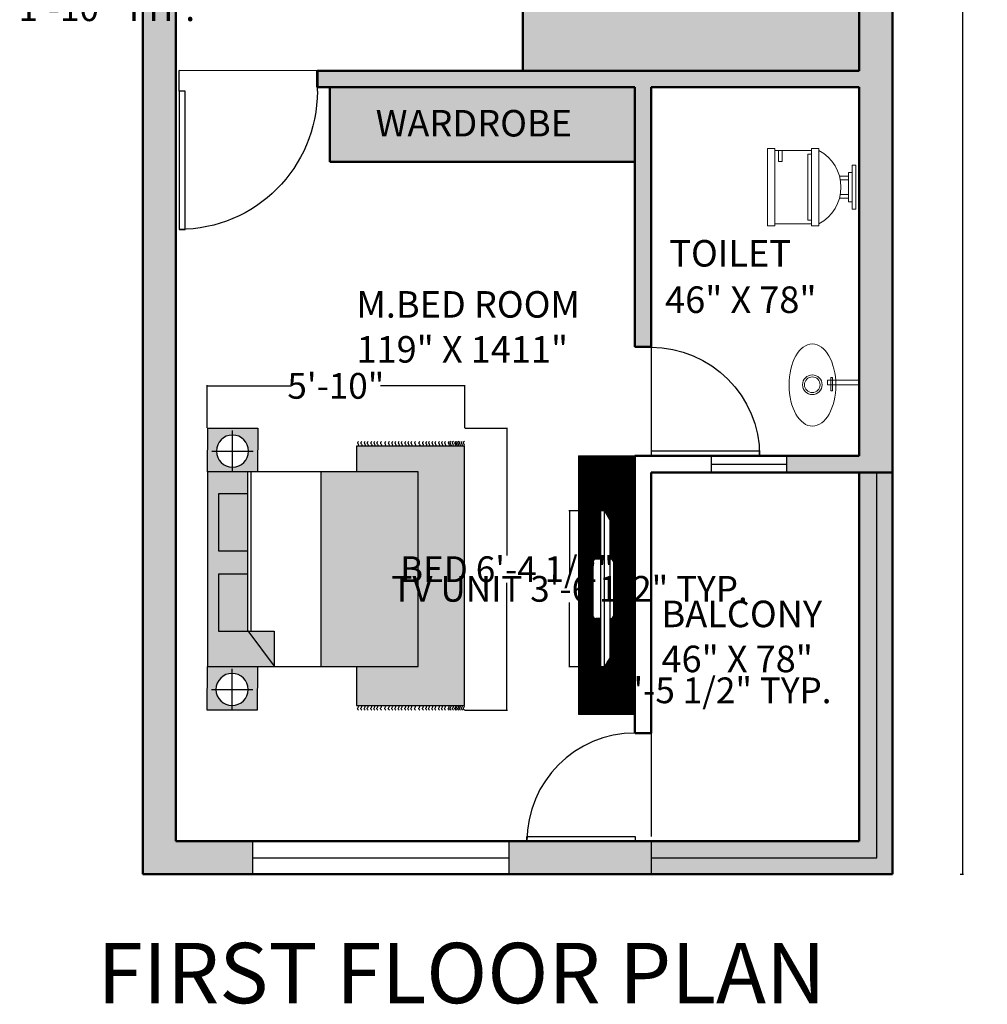
# Model space of a CAD drawing. Units: inches. Extents: x 679 to 1269, y 101 to 755.
# Tile 2 of 6: x 952 to 1216, y 102 to 370. Entities that reach past the tile are written whole.
import ezdxf

# ---------------------------------------------------------------- set-up
doc = ezdxf.new("R2010")
doc.units = ezdxf.units.IN
doc.header["$MEASUREMENT"] = 0
for name, color, linetype, lineweight in [('A-ANNO-DIMS', 2, 'Continuous', 18), ('A-ANNO-TEXT', 7, 'Continuous', 25), ('A-AREA-IDEN', 7, 'Continuous', 25), ('A-DOOR', 4, 'Continuous', 25), ('A-FLOR-FIXT', 8, 'Continuous', 18), ('A-FLOR-PATT', 8, 'Continuous', 13), ('A-FURN', 32, 'Continuous', 18), ('A-FURN-PATT', 252, 'Continuous', 13), ('A-GLAZ', 4, 'Continuous', 25), ('A-WALL', 7, 'Continuous', 50), ('A-WALL-PATT', 8, 'Continuous', 13)]:
    doc.layers.add(name, color=color, linetype=linetype, lineweight=lineweight)
doc.layers.add('furniture', color=32, linetype='Continuous')
doc.styles.get("Standard").update_dxf_attribs({"font": 'arial.ttf'})
doc.dimstyles.get("Standard").update_dxf_attribs({"dimtxt": 7, "dimasz": 0.18, "dimexe": 0.18, "dimexo": 0.0625, "dimgap": 0.09, "dimtad": 0, "dimtih": 1, "dimtoh": 1, "dimzin": 0, "dimdsep": 46, "dimlunit": 3, "dimtxsty": 'Standard', "dimcen": 0.09, "dimadec": 0, "dimazin": 0, "dimtfac": 1, "dimtofl": 0, "dimtmove": 0, "dimatfit": 3, "dimfxl": 1, "dimtolj": 1, "dimtzin": 0, "dimarcsym": 0})

# ---------------------------------------------------------------- blocks, each defined once
blk = doc.blocks.new('*U12')
for p, q in [((-10, 22), (-10, 12)), ((10, 12), (10, 22)), ((-10, 21), (-7, 21)), ((-7, 20), (-10, 20)), ((-7, 21), (-7, 20)), ((10.5, 12), (-10.5, 12)), ((-10.5, 10), (-10.5, 12)), ((9, 13), (-9, 13)), ((-9, 13), (-9, 12)), ((9, 12), (9, 13)), ((10.5, 12), (10.5, 10)), ((10.5, 10), (-10.5, 10)), ((-3, 4.4065), (-3, 2)), ((-2, 2), (-2, 4.1658)), ((2, 4.1658), (2, 2)), ((3, 2), (3, 4.4065)), ((4, 2), (-4, 2)), ((-4, 2), (-4, 1)), ((4, 1), (4, 2))]:
    blk.add_line(p, q)
for points in [[(10.5, 22), (10.5, 24), (-10.5, 24), (-10.5, 22)], [(6, 0), (6, 1), (-6, 1), (-6, 0)]]:
    blk.add_lwpolyline(points, close=True)
blk.add_arc((0, 15.3333), 11.3333, 208.0725, 331.9275)
blk = doc.blocks.new('PLASMA-LARGE')
at = {"layer": 'furniture'}
for p, q in [((-7.26, 0), (7.26, 0)), ((-21, -2.5), (21, -2.5)), ((-21, -2.5), (-21, -3.5)), ((-18.61, -1), (18.61, -1)), ((-8, -1), (-8, -0.74)), ((8, -1), (8, -0.74)), ((21, -2.5), (21, -3.5)), ((-21, -3.5), (21, -3.5)), ((-8, -3.5), (-8, -4.76)), ((8, -3.5), (8, -4.76)), ((-7.26, -5.5), (7.26, -5.5))]:
    blk.add_line(p, q, dxfattribs=at)
for centre, radius, start, end in [((-7.26, -0.74), 0.744, 90, 180), ((7.26, -0.74), 0.744, 0, 90), ((-13.97, -11.05), 11.07, 114.7602, 129.4175), ((13.97, -11.05), 11.07, 50.5825, 65.2398), ((-7.26, -4.76), 0.744, 180, 270), ((7.26, -4.76), 0.744, 270, 0)]:
    blk.add_arc(centre, radius, start, end, dxfattribs=at)
blk = doc.blocks.new('CARPET')
at = {"layer": 'furniture'}
for p, q in [((-51.53, -98.11), (-51.53, -55.12)), ((-51.53, -55.12), (-41.27, -55.12)), ((36, -55.12), (51.55, -55.12)), ((51.55, -55.12), (51.55, -98.11)), ((51.55, -98.11), (-51.53, -98.11))]:
    blk.add_line(p, q, dxfattribs=at)
for points, knots in [([(-53.37, -55.99), (-53.22, -55.8), (-52.9, -55.41), (-52.34, -55.8), (-51.89, -56.08), (-51.65, -55.91), (-51.53, -55.83)], [0, 0, 0, 0, 0.653278, 1.290138, 1.740457, 2.114451, 2.114451, 2.114451, 2.114451]), ([(-53.37, -57.26), (-53.22, -57.07), (-52.9, -56.67), (-52.34, -57.07), (-51.89, -57.35), (-51.65, -57.17), (-51.53, -57.1)], [0, 0, 0, 0, 0.653278, 1.290138, 1.740457, 2.114451, 2.114451, 2.114451, 2.114451]), ([(-53.37, -58.59), (-53.22, -58.4), (-52.9, -58.01), (-52.34, -58.4), (-51.89, -58.68), (-51.65, -58.5), (-51.53, -58.43)], [0, 0, 0, 0, 0.653278, 1.290138, 1.740457, 2.114451, 2.114451, 2.114451, 2.114451]), ([(53.37, -55.99), (53.22, -55.8), (52.9, -55.41), (52.34, -55.8), (51.89, -56.08), (51.65, -55.91), (51.53, -55.83)], [0, 0, 0, 0, 0.653278, 1.290138, 1.740457, 2.114451, 2.114451, 2.114451, 2.114451]), ([(53.37, -57.26), (53.22, -57.07), (52.9, -56.67), (52.34, -57.07), (51.89, -57.35), (51.65, -57.17), (51.53, -57.1)], [0, 0, 0, 0, 0.653278, 1.290138, 1.740457, 2.114451, 2.114451, 2.114451, 2.114451]), ([(53.37, -58.59), (53.22, -58.4), (52.9, -58.01), (52.34, -58.4), (51.89, -58.68), (51.65, -58.5), (51.53, -58.43)], [0, 0, 0, 0, 0.653278, 1.290138, 1.740457, 2.114451, 2.114451, 2.114451, 2.114451]), ([(-53.37, -59.78), (-53.22, -59.58), (-52.9, -59.19), (-52.34, -59.58), (-51.89, -59.86), (-51.65, -59.69), (-51.53, -59.61)], [0, 0, 0, 0, 0.653278, 1.290138, 1.740457, 2.114451, 2.114451, 2.114451, 2.114451]), ([(-53.37, -61.22), (-53.22, -61.02), (-52.9, -60.63), (-52.34, -61.02), (-51.89, -61.3), (-51.65, -61.13), (-51.53, -61.05)], [0, 0, 0, 0, 0.653278, 1.290138, 1.740457, 2.114451, 2.114451, 2.114451, 2.114451]), ([(-53.37, -62.44), (-53.22, -62.25), (-52.9, -61.86), (-52.34, -62.25), (-51.89, -62.53), (-51.65, -62.36), (-51.53, -62.28)], [0, 0, 0, 0, 0.653278, 1.290138, 1.740457, 2.114451, 2.114451, 2.114451, 2.114451]), ([(53.37, -59.78), (53.22, -59.58), (52.9, -59.19), (52.34, -59.58), (51.89, -59.86), (51.65, -59.69), (51.53, -59.61)], [0, 0, 0, 0, 0.653278, 1.290138, 1.740457, 2.114451, 2.114451, 2.114451, 2.114451]), ([(53.37, -61.22), (53.22, -61.02), (52.9, -60.63), (52.34, -61.02), (51.89, -61.3), (51.65, -61.13), (51.53, -61.05)], [0, 0, 0, 0, 0.653278, 1.290138, 1.740457, 2.114451, 2.114451, 2.114451, 2.114451]), ([(53.37, -62.44), (53.22, -62.25), (52.9, -61.86), (52.34, -62.25), (51.89, -62.53), (51.65, -62.36), (51.53, -62.28)], [0, 0, 0, 0, 0.653278, 1.290138, 1.740457, 2.114451, 2.114451, 2.114451, 2.114451]), ([(-53.37, -63.63), (-53.22, -63.43), (-52.9, -63.04), (-52.34, -63.43), (-51.89, -63.72), (-51.65, -63.54), (-51.53, -63.46)], [0, 0, 0, 0, 0.653278, 1.290138, 1.740457, 2.114451, 2.114451, 2.114451, 2.114451]), ([(-53.37, -65.07), (-53.22, -64.87), (-52.9, -64.48), (-52.34, -64.87), (-51.89, -65.15), (-51.65, -64.98), (-51.53, -64.9)], [0, 0, 0, 0, 0.653278, 1.290138, 1.740457, 2.114451, 2.114451, 2.114451, 2.114451]), ([(-53.37, -66.76), (-53.22, -66.56), (-52.9, -66.17), (-52.34, -66.56), (-51.89, -66.84), (-51.65, -66.67), (-51.53, -66.59)], [0, 0, 0, 0, 0.653278, 1.290138, 1.740457, 2.114451, 2.114451, 2.114451, 2.114451]), ([(53.37, -63.63), (53.22, -63.43), (52.9, -63.04), (52.34, -63.43), (51.89, -63.72), (51.65, -63.54), (51.53, -63.46)], [0, 0, 0, 0, 0.653278, 1.290138, 1.740457, 2.114451, 2.114451, 2.114451, 2.114451]), ([(53.37, -65.07), (53.22, -64.87), (52.9, -64.48), (52.34, -64.87), (51.89, -65.15), (51.65, -64.98), (51.53, -64.9)], [0, 0, 0, 0, 0.653278, 1.290138, 1.740457, 2.114451, 2.114451, 2.114451, 2.114451]), ([(53.37, -66.76), (53.22, -66.56), (52.9, -66.17), (52.34, -66.56), (51.89, -66.84), (51.65, -66.67), (51.53, -66.59)], [0, 0, 0, 0, 0.653278, 1.290138, 1.740457, 2.114451, 2.114451, 2.114451, 2.114451]), ([(-53.37, -68.2), (-53.22, -68), (-52.9, -67.61), (-52.34, -68), (-51.89, -68.28), (-51.65, -68.11), (-51.53, -68.03)], [0, 0, 0, 0, 0.653278, 1.290138, 1.740457, 2.114451, 2.114451, 2.114451, 2.114451]), ([(-53.37, -69.53), (-53.22, -69.33), (-52.9, -68.94), (-52.34, -69.33), (-51.89, -69.61), (-51.65, -69.44), (-51.53, -69.36)], [0, 0, 0, 0, 0.653278, 1.290138, 1.740457, 2.114451, 2.114451, 2.114451, 2.114451]), ([(-53.37, -70.79), (-53.22, -70.6), (-52.9, -70.21), (-52.34, -70.6), (-51.89, -70.88), (-51.65, -70.7), (-51.53, -70.63)], [0, 0, 0, 0, 0.653278, 1.290138, 1.740457, 2.114451, 2.114451, 2.114451, 2.114451]), ([(53.37, -68.2), (53.22, -68), (52.9, -67.61), (52.34, -68), (51.89, -68.28), (51.65, -68.11), (51.53, -68.03)], [0, 0, 0, 0, 0.653278, 1.290138, 1.740457, 2.114451, 2.114451, 2.114451, 2.114451]), ([(53.37, -69.53), (53.22, -69.33), (52.9, -68.94), (52.34, -69.33), (51.89, -69.61), (51.65, -69.44), (51.53, -69.36)], [0, 0, 0, 0, 0.653278, 1.290138, 1.740457, 2.114451, 2.114451, 2.114451, 2.114451]), ([(53.37, -70.79), (53.22, -70.6), (52.9, -70.21), (52.34, -70.6), (51.89, -70.88), (51.65, -70.7), (51.53, -70.63)], [0, 0, 0, 0, 0.653278, 1.290138, 1.740457, 2.114451, 2.114451, 2.114451, 2.114451]), ([(-53.37, -72.12), (-53.22, -71.93), (-52.9, -71.54), (-52.34, -71.93), (-51.89, -72.21), (-51.65, -72.04), (-51.53, -71.96)], [0, 0, 0, 0, 0.653278, 1.290138, 1.740457, 2.114451, 2.114451, 2.114451, 2.114451]), ([(-53.37, -73.31), (-53.22, -73.11), (-52.9, -72.72), (-52.34, -73.11), (-51.89, -73.4), (-51.65, -73.22), (-51.53, -73.14)], [0, 0, 0, 0, 0.653278, 1.290138, 1.740457, 2.114451, 2.114451, 2.114451, 2.114451]), ([(53.37, -72.12), (53.22, -71.93), (52.9, -71.54), (52.34, -71.93), (51.89, -72.21), (51.65, -72.04), (51.53, -71.96)], [0, 0, 0, 0, 0.653278, 1.290138, 1.740457, 2.114451, 2.114451, 2.114451, 2.114451]), ([(53.37, -73.31), (53.22, -73.11), (52.9, -72.72), (52.34, -73.11), (51.89, -73.4), (51.65, -73.22), (51.53, -73.14)], [0, 0, 0, 0, 0.653278, 1.290138, 1.740457, 2.114451, 2.114451, 2.114451, 2.114451]), ([(-53.37, -74.75), (-53.22, -74.55), (-52.9, -74.16), (-52.34, -74.55), (-51.89, -74.83), (-51.65, -74.66), (-51.53, -74.58)], [0, 0, 0, 0, 0.653278, 1.290138, 1.740457, 2.114451, 2.114451, 2.114451, 2.114451]), ([(-53.37, -75.98), (-53.22, -75.78), (-52.9, -75.39), (-52.34, -75.78), (-51.89, -76.06), (-51.65, -75.89), (-51.53, -75.81)], [0, 0, 0, 0, 0.653278, 1.290138, 1.740457, 2.114451, 2.114451, 2.114451, 2.114451]), ([(-53.37, -77.16), (-53.22, -76.96), (-52.9, -76.57), (-52.34, -76.96), (-51.89, -77.25), (-51.65, -77.07), (-51.53, -76.99)], [0, 0, 0, 0, 0.653278, 1.290138, 1.740457, 2.114451, 2.114451, 2.114451, 2.114451]), ([(-53.37, -78.6), (-53.22, -78.4), (-52.9, -78.01), (-52.34, -78.4), (-51.89, -78.68), (-51.65, -78.51), (-51.53, -78.43)], [0, 0, 0, 0, 0.653278, 1.290138, 1.740457, 2.114451, 2.114451, 2.114451, 2.114451]), ([(53.37, -74.75), (53.22, -74.55), (52.9, -74.16), (52.34, -74.55), (51.89, -74.83), (51.65, -74.66), (51.53, -74.58)], [0, 0, 0, 0, 0.653278, 1.290138, 1.740457, 2.114451, 2.114451, 2.114451, 2.114451]), ([(53.37, -75.98), (53.22, -75.78), (52.9, -75.39), (52.34, -75.78), (51.89, -76.06), (51.65, -75.89), (51.53, -75.81)], [0, 0, 0, 0, 0.653278, 1.290138, 1.740457, 2.114451, 2.114451, 2.114451, 2.114451]), ([(53.37, -77.16), (53.22, -76.96), (52.9, -76.57), (52.34, -76.96), (51.89, -77.25), (51.65, -77.07), (51.53, -76.99)], [0, 0, 0, 0, 0.653278, 1.290138, 1.740457, 2.114451, 2.114451, 2.114451, 2.114451]), ([(53.37, -78.6), (53.22, -78.4), (52.9, -78.01), (52.34, -78.4), (51.89, -78.68), (51.65, -78.51), (51.53, -78.43)], [0, 0, 0, 0, 0.653278, 1.290138, 1.740457, 2.114451, 2.114451, 2.114451, 2.114451]), ([(-53.37, -80.29), (-53.22, -80.09), (-52.9, -79.7), (-52.34, -80.09), (-51.89, -80.37), (-51.65, -80.2), (-51.53, -80.12)], [0, 0, 0, 0, 0.653278, 1.290138, 1.740457, 2.114451, 2.114451, 2.114451, 2.114451]), ([(-53.37, -81.73), (-53.22, -81.53), (-52.9, -81.14), (-52.34, -81.53), (-51.89, -81.81), (-51.65, -81.64), (-51.53, -81.56)], [0, 0, 0, 0, 0.653278, 1.290138, 1.740457, 2.114451, 2.114451, 2.114451, 2.114451]), ([(53.37, -80.29), (53.22, -80.09), (52.9, -79.7), (52.34, -80.09), (51.89, -80.37), (51.65, -80.2), (51.53, -80.12)], [0, 0, 0, 0, 0.653278, 1.290138, 1.740457, 2.114451, 2.114451, 2.114451, 2.114451]), ([(53.37, -81.73), (53.22, -81.53), (52.9, -81.14), (52.34, -81.53), (51.89, -81.81), (51.65, -81.64), (51.53, -81.56)], [0, 0, 0, 0, 0.653278, 1.290138, 1.740457, 2.114451, 2.114451, 2.114451, 2.114451]), ([(-53.37, -83.06), (-53.22, -82.86), (-52.9, -82.47), (-52.34, -82.86), (-51.89, -83.14), (-51.65, -82.97), (-51.53, -82.89)], [0, 0, 0, 0, 0.653278, 1.290138, 1.740457, 2.114451, 2.114451, 2.114451, 2.114451]), ([(-53.37, -84.18), (-53.22, -83.99), (-52.9, -83.6), (-52.34, -83.99), (-51.89, -84.27), (-51.65, -84.09), (-51.53, -84.02)], [0, 0, 0, 0, 0.653278, 1.290138, 1.740457, 2.114451, 2.114451, 2.114451, 2.114451]), ([(-53.37, -85.51), (-53.22, -85.32), (-52.9, -84.93), (-52.34, -85.32), (-51.89, -85.6), (-51.65, -85.42), (-51.53, -85.35)], [0, 0, 0, 0, 0.653278, 1.290138, 1.740457, 2.114451, 2.114451, 2.114451, 2.114451]), ([(53.37, -83.06), (53.22, -82.86), (52.9, -82.47), (52.34, -82.86), (51.89, -83.14), (51.65, -82.97), (51.53, -82.89)], [0, 0, 0, 0, 0.653278, 1.290138, 1.740457, 2.114451, 2.114451, 2.114451, 2.114451]), ([(53.37, -84.18), (53.22, -83.99), (52.9, -83.6), (52.34, -83.99), (51.89, -84.27), (51.65, -84.09), (51.53, -84.02)], [0, 0, 0, 0, 0.653278, 1.290138, 1.740457, 2.114451, 2.114451, 2.114451, 2.114451]), ([(53.37, -85.51), (53.22, -85.32), (52.9, -84.93), (52.34, -85.32), (51.89, -85.6), (51.65, -85.42), (51.53, -85.35)], [0, 0, 0, 0, 0.653278, 1.290138, 1.740457, 2.114451, 2.114451, 2.114451, 2.114451]), ([(-53.37, -86.7), (-53.22, -86.5), (-52.9, -86.11), (-52.34, -86.5), (-51.89, -86.78), (-51.65, -86.61), (-51.53, -86.53)], [0, 0, 0, 0, 0.653278, 1.290138, 1.740457, 2.114451, 2.114451, 2.114451, 2.114451]), ([(-53.37, -88.14), (-53.22, -87.94), (-52.9, -87.55), (-52.34, -87.94), (-51.89, -88.22), (-51.65, -88.05), (-51.53, -87.97)], [0, 0, 0, 0, 0.653278, 1.290138, 1.740457, 2.114451, 2.114451, 2.114451, 2.114451]), ([(-53.37, -89.36), (-53.22, -89.17), (-52.9, -88.78), (-52.34, -89.17), (-51.89, -89.45), (-51.65, -89.28), (-51.53, -89.2)], [0, 0, 0, 0, 0.653278, 1.290138, 1.740457, 2.114451, 2.114451, 2.114451, 2.114451]), ([(53.37, -86.7), (53.22, -86.5), (52.9, -86.11), (52.34, -86.5), (51.89, -86.78), (51.65, -86.61), (51.53, -86.53)], [0, 0, 0, 0, 0.653278, 1.290138, 1.740457, 2.114451, 2.114451, 2.114451, 2.114451]), ([(53.37, -88.14), (53.22, -87.94), (52.9, -87.55), (52.34, -87.94), (51.89, -88.22), (51.65, -88.05), (51.53, -87.97)], [0, 0, 0, 0, 0.653278, 1.290138, 1.740457, 2.114451, 2.114451, 2.114451, 2.114451]), ([(53.37, -89.36), (53.22, -89.17), (52.9, -88.78), (52.34, -89.17), (51.89, -89.45), (51.65, -89.28), (51.53, -89.2)], [0, 0, 0, 0, 0.653278, 1.290138, 1.740457, 2.114451, 2.114451, 2.114451, 2.114451]), ([(-53.37, -90.55), (-53.22, -90.35), (-52.9, -89.96), (-52.34, -90.35), (-51.89, -90.64), (-51.65, -90.46), (-51.53, -90.38)], [0, 0, 0, 0, 0.653278, 1.290138, 1.740457, 2.114451, 2.114451, 2.114451, 2.114451]), ([(-53.37, -91.99), (-53.22, -91.79), (-52.9, -91.4), (-52.34, -91.79), (-51.89, -92.07), (-51.65, -91.9), (-51.53, -91.82)], [0, 0, 0, 0, 0.653278, 1.290138, 1.740457, 2.114451, 2.114451, 2.114451, 2.114451]), ([(-53.37, -92.69), (-53.22, -92.48), (-52.9, -92.08), (-52.35, -92.49), (-51.89, -92.77), (-51.65, -92.6), (-51.53, -92.52)], [0, 0, 0, 0, 0.663904, 1.307406, 1.757725, 2.131719, 2.131719, 2.131719, 2.131719]), ([(-53.37, -93.61), (-53.22, -93.42), (-52.9, -93.03), (-52.34, -93.42), (-51.89, -93.7), (-51.65, -93.52), (-51.53, -93.45)], [0, 0, 0, 0, 0.653278, 1.290138, 1.740457, 2.114451, 2.114451, 2.114451, 2.114451]), ([(53.37, -90.55), (53.22, -90.35), (52.9, -89.96), (52.34, -90.35), (51.9, -90.63), (51.66, -90.47), (51.55, -90.4)], [0, 0, 0, 0, 0.653278, 1.290138, 1.740457, 2.0926, 2.0926, 2.0926, 2.0926]), ([(53.37, -91.99), (53.22, -91.79), (52.9, -91.4), (52.34, -91.79), (51.9, -92.07), (51.66, -91.91), (51.55, -91.83)], [0, 0, 0, 0, 0.653278, 1.290138, 1.740457, 2.0926, 2.0926, 2.0926, 2.0926]), ([(53.37, -92.69), (53.22, -92.49), (52.9, -92.09), (52.34, -92.49), (51.9, -92.77), (51.66, -92.61), (51.55, -92.53)], [0, 0, 0, 0, 0.656792, 1.295826, 1.746145, 2.098292, 2.098292, 2.098292, 2.098292]), ([(53.37, -93.66), (53.22, -93.46), (52.9, -93.07), (52.34, -93.46), (51.9, -93.74), (51.66, -93.58), (51.55, -93.5)], [0, 0, 0, 0, 0.653278, 1.290138, 1.740457, 2.0926, 2.0926, 2.0926, 2.0926]), ([(-53.37, -94.55), (-53.22, -94.35), (-52.9, -93.96), (-52.34, -94.35), (-51.89, -94.63), (-51.65, -94.46), (-51.53, -94.38)], [0, 0, 0, 0, 0.653278, 1.290138, 1.740457, 2.114451, 2.114451, 2.114451, 2.114451]), ([(-53.37, -95.05), (-53.22, -94.85), (-52.9, -94.46), (-52.34, -94.85), (-51.89, -95.14), (-51.65, -94.96), (-51.53, -94.88)], [0, 0, 0, 0, 0.653278, 1.290138, 1.740457, 2.114451, 2.114451, 2.114451, 2.114451]), ([(-53.37, -95.73), (-53.22, -95.54), (-52.9, -95.15), (-52.34, -95.54), (-51.89, -95.82), (-51.65, -95.65), (-51.53, -95.57)], [0, 0, 0, 0, 0.653278, 1.290138, 1.740457, 2.114451, 2.114451, 2.114451, 2.114451]), ([(-53.37, -96.38), (-53.22, -96.18), (-52.9, -95.79), (-52.34, -96.18), (-51.89, -96.47), (-51.65, -96.29), (-51.53, -96.21)], [0, 0, 0, 0, 0.653278, 1.290138, 1.740457, 2.114451, 2.114451, 2.114451, 2.114451]), ([(-53.37, -97.17), (-53.22, -96.98), (-52.9, -96.59), (-52.34, -96.98), (-51.89, -97.26), (-51.65, -97.08), (-51.53, -97.01)], [0, 0, 0, 0, 0.653278, 1.290138, 1.740457, 2.114451, 2.114451, 2.114451, 2.114451]), ([(-53.37, -97.99), (-53.22, -97.79), (-52.9, -97.4), (-52.34, -97.79), (-51.89, -98.08), (-51.65, -97.9), (-51.53, -97.82)], [0, 0, 0, 0, 0.653278, 1.290138, 1.740457, 2.114451, 2.114451, 2.114451, 2.114451]), ([(53.37, -95.78), (53.22, -95.58), (52.9, -95.19), (52.34, -95.58), (51.89, -95.86), (51.65, -95.69), (51.53, -95.61)], [0, 0, 0, 0, 0.653278, 1.290138, 1.740457, 2.114451, 2.114451, 2.114451, 2.114451]), ([(53.37, -96.43), (53.22, -96.23), (52.9, -95.84), (52.34, -96.23), (51.89, -96.51), (51.65, -96.34), (51.53, -96.26)], [0, 0, 0, 0, 0.653278, 1.290138, 1.740457, 2.114451, 2.114451, 2.114451, 2.114451]), ([(53.37, -97.22), (53.22, -97.02), (52.9, -96.63), (52.34, -97.02), (51.89, -97.3), (51.65, -97.13), (51.53, -97.05)], [0, 0, 0, 0, 0.653278, 1.290138, 1.740457, 2.114451, 2.114451, 2.114451, 2.114451]), ([(53.37, -97.99), (53.22, -97.79), (52.9, -97.4), (52.34, -97.79), (51.89, -98.08), (51.65, -97.9), (51.53, -97.82)], [0, 0, 0, 0, 0.653278, 1.290138, 1.740457, 2.114451, 2.114451, 2.114451, 2.114451]), ([(53.37, -94.59), (53.22, -94.4), (52.9, -94.01), (52.34, -94.4), (51.9, -94.68), (51.66, -94.51), (51.55, -94.44)], [0, 0, 0, 0, 0.653278, 1.290138, 1.740457, 2.0926, 2.0926, 2.0926, 2.0926]), ([(53.37, -95.1), (53.22, -94.9), (52.9, -94.51), (52.34, -94.9), (51.9, -95.18), (51.66, -95.02), (51.55, -94.94)], [0, 0, 0, 0, 0.653278, 1.290138, 1.740457, 2.0926, 2.0926, 2.0926, 2.0926])]:
    blk.add_open_spline(points, degree=3, knots=knots, dxfattribs=at)
blk = doc.blocks.new('A$C58D270C6')
at = {"layer": 'furniture'}
for p, q in [((9.09, 124.13), (9.09, 108.87)), ((1.46, 116.5), (16.73, 116.5)), ((14.97, 94.84), (24.62, 107.92)), ((24.62, 94.93), (24.62, 107.92)), ((42.08, 108), (42.08, 36)), ((14.97, 94.93), (24.62, 94.93)), ((14.97, 94.84), (14.97, 36)), ((16.22, 94.93), (16.22, 36)), ((9.25, 36), (9.25, 20.74)), ((1.62, 28.37), (16.88, 28.37))]:
    blk.add_line(p, q, dxfattribs=at)
for points in [[(18.5, 108), (18.34, 124.13), (-0.16, 124.13), (0, 108)], [(0, 108), (77.91, 108), (77.91, 36), (0, 36)], [(4.09, 94.93), (14.97, 94.93), (14.97, 73.83), (4.09, 73.83)], [(4.09, 65.23), (14.97, 65.23), (14.97, 44.13), (4.09, 44.13)], [(18.65, 19.87), (18.5, 36), (0, 36), (0.16, 19.87)]]:
    blk.add_lwpolyline(points, close=True, dxfattribs=at)
for centre in [(9.09, 116.5), (9.25, 28.37)]:
    blk.add_circle(centre, 5.95, dxfattribs=at)
at = {"layer": 'furniture', "xscale": 0.9312884925094044, "yscale": 0.9312884925094044, "zscale": 0.9312884925094044, "rotation": 90}
blk.add_blockref('CARPET', (3.79, 74.47), dxfattribs=at)
blk = doc.blocks.new('*U4')
for p, q in [((0, 0), (0, -6)), ((40, 0), (40, -6))]:
    blk.add_line(p, q)
blk.add_lwpolyline([(0, 0), (0, 40), (1.75, 40), (1.75, 0)], close=True)
blk.add_arc((0, 0), 40, 0, 90)
blk = doc.blocks.new('*D16')
at = {"layer": 'A-ANNO-DIMS', "color": 0, "lineweight": -2, "transparency": 16777216}
for p, q in [((1208.37, 737.73), (1209.33, 737.73)), ((1209.15, 737.55), (1209.15, 441.39)), ((1209.15, 137.91), (1209.15, 434.07)), ((1208.37, 137.73), (1209.33, 137.73))]:
    blk.add_line(p, q, dxfattribs=at)
at = {"layer": 'A-ANNO-DIMS', "color": 0, "transparency": 16777216}
for points in [[(1209.12, 737.55), (1209.18, 737.55), (1209.15, 737.73)], [(1209.12, 137.91), (1209.18, 137.91), (1209.15, 137.73)]]:
    blk.add_solid(points, dxfattribs=at)
at = {"layer": 'Defpoints', "color": 0, "transparency": 16777216}
for p in [(1208.3, 737.73), (1208.3, 137.73), (1209.15, 137.73)]:
    blk.add_point(p, dxfattribs=at)
at = {"layer": 'A-ANNO-DIMS', "color": 0, "transparency": 16777216, "insert": (1209.15, 437.73), "char_height": 7, "attachment_point": 5}
blk.add_mtext("\\A1;50'", dxfattribs=at)
blk = doc.blocks.new('WASHBASIN')
for p, q in [((8.57, 12.49), (0, 12.49)), ((8.57, 11.25), (0, 11.25)), ((7.24, 9.62), (7.23, 13.28)), ((7.23, 13.28), (7.63, 13.28)), ((7.63, 13.28), (7.65, 9.63)), ((8.57, 11.25), (8.57, 12.49)), ((7.24, 9.62), (7.65, 9.63))]:
    blk.add_line(p, q)
for radius in [2.67, 2.13]:
    blk.add_circle((12.7, 11.27), radius)
at = {"extrusion": (0, 0, -1)}
blk.add_ellipse((12.66, 11.2), major_axis=(0.03, 11.2), ratio=0.56899, dxfattribs=at)
blk = doc.blocks.new('*D23')
at = {"layer": 'A-ANNO-DIMS', "color": 0, "lineweight": -2, "transparency": 16777216}
for p, q in [((1073.57, 259.1), (1085.2, 259.1)), ((1085.02, 258.92), (1085.02, 224.44)), ((1085.02, 182.55), (1085.02, 217.02)), ((1073.57, 182.37), (1085.2, 182.37))]:
    blk.add_line(p, q, dxfattribs=at)
at = {"layer": 'A-ANNO-DIMS', "color": 0, "transparency": 16777216}
for points in [[(1084.99, 258.92), (1085.05, 258.92), (1085.02, 259.1)], [(1084.99, 182.55), (1085.05, 182.55), (1085.02, 182.37)]]:
    blk.add_solid(points, dxfattribs=at)
at = {"layer": 'Defpoints', "color": 0, "transparency": 16777216}
for p in [(1073.51, 259.1), (1073.51, 182.37), (1085.02, 182.37)]:
    blk.add_point(p, dxfattribs=at)
at = {"layer": 'A-ANNO-DIMS', "color": 0, "transparency": 16777216, "insert": (1085.02, 220.73), "char_height": 7, "attachment_point": 5}
blk.add_mtext('\\A1;BED 6\'-4 1/2"', dxfattribs=at)
blk = doc.blocks.new('*D24')
at = {"layer": 'A-ANNO-DIMS', "color": 0, "lineweight": -2, "transparency": 16777216}
for p, q in [((1003.39, 259.16), (1003.39, 270.79)), ((1003.57, 270.61), (1026.34, 270.61)), ((1073.33, 270.61), (1050.56, 270.61)), ((1073.51, 259.16), (1073.51, 270.79))]:
    blk.add_line(p, q, dxfattribs=at)
at = {"layer": 'A-ANNO-DIMS', "color": 0, "transparency": 16777216}
for points in [[(1003.57, 270.64), (1003.57, 270.58), (1003.39, 270.61)], [(1073.33, 270.64), (1073.33, 270.58), (1073.51, 270.61)]]:
    blk.add_solid(points, dxfattribs=at)
at = {"layer": 'Defpoints', "color": 0, "transparency": 16777216}
for p in [(1073.51, 270.61), (1003.39, 259.1), (1073.51, 259.1)]:
    blk.add_point(p, dxfattribs=at)
at = {"layer": 'A-ANNO-DIMS', "color": 0, "transparency": 16777216, "insert": (1038.45, 270.61), "char_height": 7, "attachment_point": 5}
blk.add_mtext('\\A1;5\'-10"', dxfattribs=at)
blk = doc.blocks.new('*D27')
at = {"layer": 'A-ANNO-DIMS', "color": 0, "lineweight": -2, "transparency": 16777216}
for p, q in [((854.14, 376.61), (854.14, 373.18)), ((876.23, 376.61), (876.23, 373.18)), ((854.32, 373.36), (876.05, 373.36)), ((876.23, 373.36), (876.41, 373.36))]:
    blk.add_line(p, q, dxfattribs=at)
at = {"layer": 'A-ANNO-DIMS', "color": 0, "transparency": 16777216}
for points in [[(854.32, 373.39), (854.32, 373.33), (854.14, 373.36)], [(876.05, 373.39), (876.05, 373.33), (876.23, 373.36)]]:
    blk.add_solid(points, dxfattribs=at)
at = {"layer": 'Defpoints', "color": 0, "transparency": 16777216}
for p in [(854.14, 376.67), (876.23, 376.67), (876.23, 373.36)]:
    blk.add_point(p, dxfattribs=at)
at = {"layer": 'A-ANNO-DIMS', "color": 0, "transparency": 16777216, "insert": (940.47, 373.36), "char_height": 7, "attachment_point": 5}
blk.add_mtext('\\A1;SOFA 1-SEATER 1\'-10" TYP.', dxfattribs=at)
blk = doc.blocks.new('*D33')
at = {"layer": 'A-ANNO-DIMS', "color": 0, "lineweight": -2, "transparency": 16777216}
for p, q in [((1108.37, 236.61), (1101.88, 236.61)), ((1102.06, 236.43), (1102.06, 219.09)), ((1102.06, 194.32), (1102.06, 211.66)), ((1108.37, 194.14), (1101.88, 194.14))]:
    blk.add_line(p, q, dxfattribs=at)
at = {"layer": 'A-ANNO-DIMS', "color": 0, "transparency": 16777216}
for points in [[(1102.03, 236.43), (1102.09, 236.43), (1102.06, 236.61)], [(1102.03, 194.32), (1102.09, 194.32), (1102.06, 194.14)]]:
    blk.add_solid(points, dxfattribs=at)
at = {"layer": 'Defpoints', "color": 0, "transparency": 16777216}
for p in [(1108.43, 236.61), (1102.06, 194.14), (1108.43, 194.14)]:
    blk.add_point(p, dxfattribs=at)
at = {"layer": 'A-ANNO-DIMS', "color": 0, "transparency": 16777216, "insert": (1102.06, 215.38), "char_height": 7, "attachment_point": 5}
blk.add_mtext('\\A1;TV UNIT 3\'-6 1/2" TYP.', dxfattribs=at)
blk = doc.blocks.new('*D34')
at = {"layer": 'A-ANNO-DIMS', "color": 0, "lineweight": -2, "transparency": 16777216}
for p, q in [((1108.43, 194.08), (1108.43, 187.59)), ((1114, 194.08), (1114, 187.59)), ((1108.61, 187.77), (1113.82, 187.77)), ((1114, 187.77), (1114.18, 187.77))]:
    blk.add_line(p, q, dxfattribs=at)
at = {"layer": 'A-ANNO-DIMS', "color": 0, "transparency": 16777216}
for points in [[(1108.61, 187.8), (1108.61, 187.74), (1108.43, 187.77)], [(1113.82, 187.8), (1113.82, 187.74), (1114, 187.77)]]:
    blk.add_solid(points, dxfattribs=at)
at = {"layer": 'Defpoints', "color": 0, "transparency": 16777216}
for p in [(1108.43, 194.14), (1114, 194.14), (1114, 187.77)]:
    blk.add_point(p, dxfattribs=at)
at = {"layer": 'A-ANNO-DIMS', "color": 0, "transparency": 16777216, "insert": (1143.76, 187.77), "char_height": 7, "attachment_point": 5}
blk.add_mtext('\\A1;0\'-5 1/2" TYP.', dxfattribs=at)

msp = doc.modelspace()

# ---------------------------------------------------------------- hatches: boundary and pattern name
at = {"layer": 'A-FLOR-PATT'}
h = msp.add_hatch(dxfattribs=at)
h.set_pattern_fill('ANSI31', color=256)
h.paths.add_polyline_path([(1119.805, 251.542), (1104.539, 251.542), (1104.539, 181.227), (1119.805, 181.227)])
h.paths.add_polyline_path([(1111.468, 194.139), (1110.457, 194.139), (1110.457, 207.286), (1109.187, 207.286, -0.4142136), (1108.434, 208.038), (1108.434, 222.713, -0.4142136), (1109.187, 223.466), (1110.457, 223.466), (1110.457, 236.613), (1111.468, 236.613, -0.0640419), (1112.985, 234.194), (1112.985, 223.466), (1113.243, 223.466, -0.4142136), (1113.996, 222.713), (1113.996, 208.038, -0.4142136), (1113.243, 207.286), (1112.985, 207.286), (1112.985, 196.558, -0.0640419)], flags=16)
h.paths.add_polyline_path([(794.414, 488.811), (775.786, 488.811), (775.786, 449.729), (775.786, 418.496), (794.414, 418.496)])
h.paths.add_polyline_path([(785.134, 431.408), (784.123, 431.408, -0.0640419), (782.606, 433.827), (782.606, 444.555), (782.347, 444.555, -0.4142136), (781.595, 445.308), (781.595, 459.983, -0.4142136), (782.347, 460.736), (782.606, 460.736), (782.606, 471.463, -0.0640419), (784.123, 473.882), (785.134, 473.882), (785.134, 460.736), (786.404, 460.736, -0.4142136), (787.157, 459.983), (787.157, 445.308, -0.4142136), (786.404, 444.555), (785.134, 444.555)], flags=16)
at = {"layer": 'A-FURN-PATT'}
h = msp.add_hatch(color=256, dxfattribs=at)
h.dxf.hatch_style = 1
h.paths.add_polyline_path([(1119.805, 351.854), (1036.785, 351.854), (1036.785, 331.601), (1119.805, 331.601)])
at = {"layer": 'A-GLAZ'}
h = msp.add_hatch(color=256, dxfattribs=at)
h.dxf.hatch_style = 1
h.paths.add_polyline_path([(994.931, 583.729), (1053.502, 583.729), (1053.502, 588.883), (1053.502, 623.243), (1053.502, 645.329), (1049.002, 645.329), (1049.002, 588.229), (994.931, 588.229), (994.931, 674.229), (1053.502, 674.229), (1053.502, 678.729), (994.931, 678.729), (994.931, 728.729), (1180.931, 728.729), (1180.931, 356.354), (1033.405, 356.354), (1033.405, 351.854), (1119.805, 351.854), (1119.805, 281.2), (1124.305, 281.2), (1124.305, 351.854), (1180.931, 351.854), (1180.931, 251.542), (1161.199, 251.542), (1161.199, 247.042), (1189.931, 247.042), (1189.931, 737.729), (985.931, 737.729), (985.931, 137.729), (1015.759, 137.729), (1015.759, 146.729), (994.931, 146.729)])
h.paths.add_polyline_path([(1185.698, 247.042), (1180.931, 247.042), (1180.931, 146.729), (1124.305, 146.729), (1124.305, 142.229), (1185.698, 142.229)], flags=0)
h.paths.add_polyline_path([(1189.931, 247.042), (1185.698, 247.042), (1185.698, 142.229), (1124.305, 142.229), (1124.305, 137.729), (1189.931, 137.729)], flags=17)
at = {"layer": 'A-WALL-PATT'}
h = msp.add_hatch(color=256, dxfattribs=at)
h.dxf.hatch_style = 1
h.paths.add_polyline_path([(1189.931, 737.729), (985.931, 737.729), (985.931, 137.729), (1015.759, 137.729), (1015.759, 146.729), (994.931, 146.729), (994.931, 583.729), (1053.502, 583.729), (1053.502, 645.329), (1049.002, 645.329), (1049.002, 588.229), (994.931, 588.229), (994.931, 674.229), (1012.305, 674.229), (1012.305, 678.729), (994.931, 678.729), (994.931, 728.729), (1053.502, 728.729), (1053.502, 678.729), (1053.502, 674.229), (1049.002, 674.229), (1049.002, 645.329), (1053.502, 645.329), (1053.502, 583.729), (994.931, 583.729), (994.931, 146.729), (1180.931, 146.729), (1180.931, 247.042), (1124.305, 247.042), (1124.305, 176.159), (1119.805, 176.159), (1119.805, 181.227), (1104.539, 181.227), (1104.539, 251.542), (1119.805, 251.542), (1124.238, 251.542), (1124.238, 281.2), (1119.805, 281.2), (1119.805, 331.601), (1036.785, 331.601), (1036.785, 351.854), (1033.393, 351.854), (1033.393, 356.354), (1033.405, 356.354), (1089.362, 356.354), (1089.362, 507.268), (1180.931, 507.268), (1180.931, 356.354), (1089.362, 356.354), (1033.405, 356.354), (1033.405, 351.854), (1119.805, 351.854), (1119.805, 281.2), (1124.305, 281.2), (1124.305, 351.854), (1180.931, 351.854), (1180.931, 251.542), (1161.199, 251.542), (1161.199, 247.042), (1189.931, 247.042)], flags=17)
h.paths.add_polyline_path([(1087.931, 548.661), (1087.931, 583.729), (1087.862, 588.229), (1087.862, 583.729), (1087.931, 583.729), (1150.34, 583.729), (1150.34, 548.661)], flags=0)
h.paths.add_polyline_path([(1161.61, 599.984, -0.2489628), (1161.61, 610.804), (1161.61, 612.705, -0.611129), (1176.66, 612.705), (1176.66, 610.804, -0.2489628), (1176.66, 599.984)], flags=0)
h.paths.add_polyline_path([(1064.382, 534.011), (1064.382, 508.83), (1050.613, 508.83), (1050.613, 534.011)], flags=0)
h.paths.add_polyline_path([(1153.405, 653.658), (1150.32, 653.658), (1150.32, 654.172), (1137.85, 654.172), (1137.85, 653.658), (1134.765, 653.658), (1134.765, 669.599), (1136.307, 669.599), (1136.307, 671.141), (1131.356, 671.141), (1131.356, 669.599), (1132.898, 669.599), (1132.898, 653.658), (1129.813, 653.658), (1129.813, 654.172), (1117.343, 654.172), (1117.343, 653.658), (1114.258, 653.658), (1114.258, 669.599), (1115.801, 669.599), (1115.801, 671.141), (1112.147, 671.141), (1112.147, 669.599), (1113.69, 669.599), (1113.69, 653.658), (1110.605, 653.658), (1110.605, 654.172), (1098.135, 654.172), (1098.135, 653.658), (1095.05, 653.658), (1095.05, 669.599), (1095.05, 671.141), (1096.592, 671.141), (1112.147, 671.141), (1115.801, 671.141), (1131.356, 671.141), (1136.307, 671.141), (1151.862, 671.141), (1153.405, 671.141), (1153.405, 669.599)], flags=0)
h.paths.add_polyline_path([(1037.949, 548.144), (1037.949, 541.332), (1012.214, 541.332), (1012.971, 540.906), (1036.813, 540.906), (1036.813, 432.764), (1012.971, 432.764), (1006.159, 428.933), (999.347, 428.933), (999.347, 544.738), (1002.753, 544.738), (1002.753, 548.144)], flags=0)
h.paths.add_polyline_path([(1037.949, 550.347), (999.347, 550.347), (999.347, 579.213), (1037.949, 579.213)], flags=0)
h.paths.add_polyline_path([(1064.382, 465.7), (1064.382, 440.519), (1050.613, 440.519), (1050.613, 465.7)], flags=0)
h.paths.add_polyline_path([(1146.082, 678.097), (1096.893, 678.097), (1096.893, 698.607), (1104.314, 698.607), (1104.314, 717.374), (1096.049, 717.453), (1096.049, 726.931), (1104.314, 726.852), (1141.204, 726.852), (1149.469, 726.772), (1149.469, 717.294), (1141.204, 717.374), (1141.204, 698.607), (1146.082, 698.607)], flags=0)
h.paths.add_polyline_path([(1189.931, 737.729), (985.931, 737.729), (985.931, 137.729), (1015.759, 137.729), (1015.759, 146.729), (994.931, 146.729), (994.931, 583.729), (1053.502, 583.729), (1053.502, 645.329), (1049.002, 645.329), (1049.002, 588.229), (994.931, 588.229), (994.931, 674.229), (1012.305, 674.229), (1012.305, 678.729), (994.931, 678.729), (994.931, 728.729), (1053.502, 728.729), (1053.502, 674.229), (1049.002, 674.229), (1049.002, 645.329), (1053.502, 645.329), (1053.502, 583.729), (994.931, 583.729), (994.931, 146.729), (1180.931, 146.729), (1180.931, 247.042), (1124.305, 247.042), (1124.305, 176.159), (1119.805, 176.159), (1119.805, 181.227), (1104.539, 181.227), (1104.539, 251.542), (1119.805, 251.542), (1124.238, 251.542), (1124.238, 281.2), (1119.805, 281.2), (1119.805, 331.601), (1036.785, 331.601), (1036.785, 351.854), (1033.393, 351.854), (1033.393, 356.354), (1089.362, 356.354), (1089.362, 507.268), (1180.931, 507.268), (1180.931, 356.354), (1033.405, 356.354), (1033.405, 351.854), (1119.805, 351.854), (1119.805, 281.2), (1124.305, 281.2), (1124.305, 351.854), (1180.931, 351.854), (1180.931, 251.542), (1161.199, 251.542), (1161.199, 247.042), (1189.931, 247.042)], flags=17)
h.paths.add_polyline_path([(1087.931, 583.729), (1087.862, 583.729), (1087.862, 588.229), (1087.862, 588.883), (1087.862, 596.11), (1152.762, 596.11), (1158.171, 599.984), (1161.61, 599.984, -0.2489628), (1161.61, 610.804), (1161.61, 612.705, -0.611129), (1176.66, 612.705), (1176.66, 610.804, -0.2489628), (1176.66, 599.984), (1161.61, 599.984), (1158.171, 599.984), (1152.762, 596.11), (1087.862, 596.11), (1087.862, 588.883), (1087.862, 588.229), (1087.931, 583.729), (1150.34, 583.729), (1150.34, 548.661), (1087.931, 548.661)], flags=0)
h.paths.add_polyline_path([(1087.931, 583.729), (1087.862, 588.229), (1087.862, 583.729), (1150.34, 583.729), (1150.34, 548.661), (1087.931, 548.661)], flags=0)
h.paths.add_polyline_path([(1161.61, 610.804), (1161.61, 612.705, -0.611129), (1176.66, 612.705), (1176.66, 610.804, -0.2489628), (1176.66, 599.984), (1176.66, 610.804, 0.4904831), (1161.61, 610.804), (1161.61, 599.984, -0.2489628)], flags=0)
h = msp.add_hatch(color=256, dxfattribs=at)
h.dxf.hatch_style = 1
h.paths.add_polyline_path([(1180.931, 507.268), (1089.362, 507.268), (1089.362, 356.354), (1180.931, 356.354)])
h.paths.add_polyline_path([(1037.949, 416.536), (999.347, 416.536), (999.347, 387.67), (1037.949, 387.67)])
h.paths.add_polyline_path([(1037.949, 579.213), (999.347, 579.213), (999.347, 550.347), (1037.949, 550.347)])
h.paths.add_polyline_path([(1064.382, 465.7), (1050.613, 465.7), (1050.613, 440.519), (1064.382, 440.519)])
h.paths.add_polyline_path([(1064.382, 534.011), (1050.613, 534.011), (1050.613, 508.83), (1064.382, 508.83)])
h.paths.add_polyline_path([(1017.114, 194.268), (1003.506, 194.268), (1003.391, 182.402), (1010.195, 182.402), (1010.195, 183.635, -0.4142136), (1005.815, 188.015, -1), (1014.576, 188.015, -0.4142136), (1010.195, 183.635), (1010.195, 182.402), (1017, 182.402)])
h.paths.add_polyline_path([(1014.691, 252.849, -0.4142136), (1010.31, 248.468), (1010.31, 247.235), (1017.114, 247.235), (1017.229, 259.102), (1003.62, 259.102), (1003.506, 247.235), (1010.31, 247.235), (1010.31, 248.468, -0.4142136), (1005.929, 252.849, -1)])
h.paths.add_polyline_path([(1104.314, 726.852), (1096.049, 726.931), (1096.049, 722.192), (1096.908, 722.192, -1), (1103.01, 722.192, -1), (1096.908, 722.192), (1096.049, 722.192), (1096.049, 717.453), (1104.314, 717.374)])
h.paths.add_polyline_path([(1149.469, 726.772), (1141.204, 726.852), (1141.204, 722.113), (1142.063, 722.113, -1), (1148.165, 722.113, -1), (1142.063, 722.113), (1141.204, 722.113), (1141.204, 717.374), (1149.469, 717.294)])
h.paths.add_polyline_path([(826.598, 726.852), (818.333, 726.931), (818.333, 722.192), (819.192, 722.192, -1), (825.294, 722.192, -1), (819.192, 722.192), (818.333, 722.192), (818.333, 717.453), (826.598, 717.374)])
h.paths.add_polyline_path([(871.752, 726.772), (863.487, 726.852), (863.487, 722.113), (864.346, 722.113, -1), (870.448, 722.113, -1), (864.346, 722.113), (863.487, 722.113), (863.487, 717.374), (871.752, 717.294)])
h = msp.add_hatch(color=256, dxfattribs=at)
h.dxf.hatch_style = 1
h.paths.add_polyline_path([(1060.816, 247.235), (1034.46, 247.235), (1034.46, 194.268), (1060.816, 194.268)])
h.paths.add_polyline_path([(1014.569, 203.882), (1006.518, 203.882), (1006.518, 219.402), (1014.521, 219.402), (1014.521, 225.734), (1006.518, 225.734), (1006.518, 241.254), (1014.521, 241.254), (1014.521, 247.235), (1003.506, 247.235), (1003.506, 194.268), (1021.615, 194.268), (1021.615, 194.326)])
h.paths.add_polyline_path([(863.487, 705.293), (826.598, 705.293), (826.598, 686.937), (863.487, 686.937)])
h.paths.add_polyline_path([(833.293, 724.754), (844.102, 724.754), (844.102, 719.18), (848.513, 719.18), (848.513, 724.754), (859.322, 724.754), (859.322, 719.18), (863.487, 719.18), (863.487, 726.852), (826.598, 726.852), (826.598, 714.239), (826.637, 714.239), (833.293, 719.147)])
h.paths.add_polyline_path([(844.102, 724.754), (833.293, 724.754), (833.293, 719.18), (844.102, 719.18)], flags=17)
h.paths.add_polyline_path([(859.322, 724.754), (848.513, 724.754), (848.513, 719.18), (859.322, 719.18)], flags=17)
h.paths.add_polyline_path([(1014.521, 219.402), (1006.518, 219.402), (1006.518, 203.882), (1014.521, 203.882)], flags=17)
h.paths.add_polyline_path([(1014.521, 241.254), (1006.518, 241.254), (1006.518, 225.734), (1014.521, 225.734)], flags=17)
h = msp.add_hatch(color=256, dxfattribs=at)
h.dxf.hatch_style = 1
h.paths.add_polyline_path([(833.293, 719.147), (826.637, 714.239), (833.293, 714.239)])
h.paths.add_polyline_path([(868.365, 698.607), (863.487, 698.607), (863.487, 686.937), (826.598, 686.937), (826.598, 698.607), (819.177, 698.607), (819.177, 678.097), (868.365, 678.097)])
h.paths.add_polyline_path([(1021.615, 203.882), (1014.569, 203.882), (1021.615, 194.326)])
h.paths.add_polyline_path([(1073.509, 254.238), (1044.06, 254.238), (1044.06, 247.235), (1060.816, 247.235), (1060.816, 194.268), (1044.06, 194.268), (1044.06, 183.613), (1073.509, 183.613)])
h = msp.add_hatch(color=256, dxfattribs=at)
h.dxf.hatch_style = 1
h.paths.add_polyline_path([(1185.698, 247.042), (1180.931, 247.042), (1180.931, 146.729), (1124.305, 146.729), (1124.305, 142.229), (1185.698, 142.229)])
h = msp.add_hatch(color=256, dxfattribs=at)
h.dxf.hatch_style = 1
h.paths.add_polyline_path([(1124.305, 146.729), (1119.891, 146.729), (1090.462, 146.729), (1085.655, 146.729), (1085.655, 137.729), (1124.305, 137.729)])

# ---------------------------------------------------------------- linework, layer by layer
at = {"layer": 'A-FURN'}
for p, q in [((1119.805, 251.542), (1104.539, 251.542)), ((1104.539, 251.542), (1104.539, 181.227)), ((1104.539, 181.227), (1119.805, 181.227))]:
    msp.add_line(p, q, dxfattribs=at)
at = {"layer": 'A-GLAZ'}
for p, q in [((1033.393, 356.354), (995.785, 356.434)), ((1124.238, 281.095), (1124.238, 251.542)), ((1140.611, 251.542), (1140.611, 247.042)), ((1161.199, 251.542), (1140.611, 251.542)), ((1140.611, 251.542), (1140.611, 249.292)), ((1140.611, 249.292), (1161.199, 249.292)), ((1161.199, 247.042), (1161.199, 251.542)), ((1140.611, 247.042), (1161.199, 247.042)), ((1185.698, 142.229), (1185.698, 247.042)), ((1124.305, 176.159), (1124.305, 148.017)), ((1015.759, 146.729), (1015.759, 137.729)), ((1085.655, 146.729), (1015.759, 146.729)), ((1015.759, 146.729), (1015.759, 142.229)), ((1085.655, 137.729), (1085.655, 146.729)), ((1124.305, 146.729), (1124.305, 137.729)), ((1015.759, 142.229), (1085.655, 142.229)), ((1124.305, 142.229), (1185.698, 142.229)), ((1015.759, 137.729), (1085.655, 137.729))]:
    msp.add_line(p, q, dxfattribs=at)
at = {"layer": 'A-WALL'}
for p, q in [((985.931, 137.729), (985.931, 737.729)), ((1189.931, 737.729), (1189.931, 137.729)), ((1180.931, 728.729), (1180.931, 356.354)), ((994.931, 146.729), (994.931, 583.729)), ((1089.362, 507.268), (1089.362, 356.354)), ((1180.931, 507.268), (1180.931, 356.354)), ((1033.393, 356.354), (1180.931, 356.354)), ((1033.393, 351.854), (1033.393, 356.354)), ((1033.405, 356.354), (1033.405, 351.854)), ((1180.931, 356.354), (1089.362, 356.354)), ((1033.393, 351.854), (1119.805, 351.854)), ((1036.785, 331.601), (1036.785, 351.854)), ((1119.805, 281.2), (1119.805, 351.854)), ((1124.305, 281.2), (1124.305, 351.854)), ((1124.305, 351.854), (1180.931, 351.854)), ((1180.931, 351.854), (1180.931, 251.542)), ((1119.805, 336.585), (1119.805, 336.585)), ((1119.805, 331.601), (1036.785, 331.601)), ((1119.805, 281.2), (1124.305, 281.2)), ((1119.805, 251.542), (1180.931, 251.542)), ((1119.805, 176.159), (1119.805, 251.542)), ((1124.305, 176.159), (1124.305, 247.042)), ((1124.305, 247.042), (1189.931, 247.042)), ((1180.931, 247.042), (1180.931, 146.729)), ((1124.305, 176.159), (1119.891, 176.159)), ((1180.931, 146.729), (994.931, 146.729)), ((1189.931, 137.729), (985.931, 137.729))]:
    msp.add_line(p, q, dxfattribs=at)

# ---------------------------------------------------------------- block references
at = {"layer": 'A-DOOR'}
for p, xscale, yscale, zscale, rotation in [((995.785, 350.791), -0.9405013235413704, 0.9405013235413704, 0.9405013235413704, 180), ((1124.238, 251.542), -0.7388186783790639, 0.7388186783790639, 0.7388186783790639, 270), ((1119.891, 146.729), 0.7357335818395229, 0.7357335818395229, 0.7357335818395229, 90.00000000000003)]:
    msp.add_blockref('*U4', p, dxfattribs=dict(at, xscale=xscale, yscale=yscale, zscale=zscale, rotation=rotation))
at = {"layer": 'A-FLOR-FIXT', "xscale": -1, "rotation": 90.00000000000007}
msp.add_blockref('*U12', (1179.951, 324.671), dxfattribs=at)
at = {"layer": 'A-FLOR-FIXT', "extrusion": (0, 0, -1), "zscale": -1}
msp.add_blockref('WASHBASIN', (-1180.844, 259.642), dxfattribs=at)
at = {"layer": 'A-FURN'}
for name, p, xscale, yscale, zscale, rotation in [('A$C58D270C6', (1003.505, 273.718), -0.7356472986026626, 0.7356472986026626, 0.7356472986026626, 180), ('PLASMA-LARGE', (1113.996, 215.376), 1.011294184530666, 1.011294184530666, 1.011294184530666, 270)]:
    msp.add_blockref(name, p, dxfattribs=dict(at, xscale=xscale, yscale=yscale, zscale=zscale, rotation=rotation))

# ---------------------------------------------------------------- texts
at = {"layer": 'A-ANNO-TEXT'}
msp.add_text('FIRST FLOOR PLAN', height=16.42699, dxfattribs=at).set_placement((973.539, 102.637))
at = {"layer": 'A-AREA-IDEN'}
for s, height, p in [('WARDROBE', 7.213, (1049.289, 338.458)), ('TOILET', 7.213, (1129.229, 303.069)), ('46" X 78"', 7.213, (1128.069, 290.448)), ('M.BED ROOM', 7.213, (1044.06, 289.174)), ('119" X 1411"', 7.21303, (1044.06, 276.934)), ('BALCONY', 7.213, (1127.088, 204.951)), ('46" X 78"', 7.213, (1127.088, 192.711))]:
    msp.add_text(s, height=height, dxfattribs=at).set_placement(p)

# ---------------------------------------------------------------- dimensions: what is measured, and where the dimension line sits
at = {"layer": 'A-ANNO-DIMS'}
dim = msp.add_linear_dim(base=(1209.153, 137.729), p1=(1208.303, 737.729), p2=(1208.303, 137.729), angle=90, dimstyle='Standard', override={"dimclrd": 0, "dimclre": 0, "dimclrt": 0}, dxfattribs=at)
dim.commit()
dim.dimension.update_dxf_attribs({"geometry": '*D16', "text_midpoint": (1209.153, 437.729)})
for base, p1, p2, text, picture, middle in [((876.227, 373.358), (854.135, 376.671), (876.227, 376.671), 'SOFA 1-SEATER <> TYP.', '*D27', (940.473, 373.358)), ((1113.996, 187.768), (1108.434, 194.139), (1113.996, 194.139), '<> TYP.', '*D34', (1143.756, 187.768))]:
    dim = msp.add_linear_dim(base=base, p1=p1, p2=p2, text=text, dimstyle='Standard', override={"dimdec": 1, "dimrnd": 0, "dimzin": 1, "dimlunit": 4, "dimfrac": 2}, dxfattribs=at)
    dim.commit()
    dim.dimension.update_dxf_attribs({"geometry": picture, "text_midpoint": middle})
dim = msp.add_linear_dim(base=(1073.509, 270.612), p1=(1003.391, 259.102), p2=(1073.509, 259.102), dimstyle='Standard', override={"dimdec": 1, "dimrnd": 0, "dimzin": 1, "dimlunit": 4, "dimfrac": 2}, dxfattribs=at)
dim.commit()
dim.dimension.update_dxf_attribs({"geometry": '*D24', "text_midpoint": (1038.45, 270.612)})
for base, p1, p2, text, picture, middle in [((1085.019, 182.366), (1073.509, 259.102), (1073.509, 182.366), 'BED <>', '*D23', (1085.019, 220.734)), ((1102.063, 194.139), (1108.434, 236.613), (1108.434, 194.139), 'TV UNIT <> TYP.', '*D33', (1102.063, 215.376))]:
    dim = msp.add_linear_dim(base=base, p1=p1, p2=p2, angle=270, text=text, dimstyle='Standard', override={"dimdec": 1, "dimrnd": 0, "dimzin": 1, "dimlunit": 4, "dimfrac": 2}, dxfattribs=at)
    dim.commit()
    dim.dimension.update_dxf_attribs({"geometry": picture, "text_midpoint": middle})

doc.saveas('drawing.dxf')
